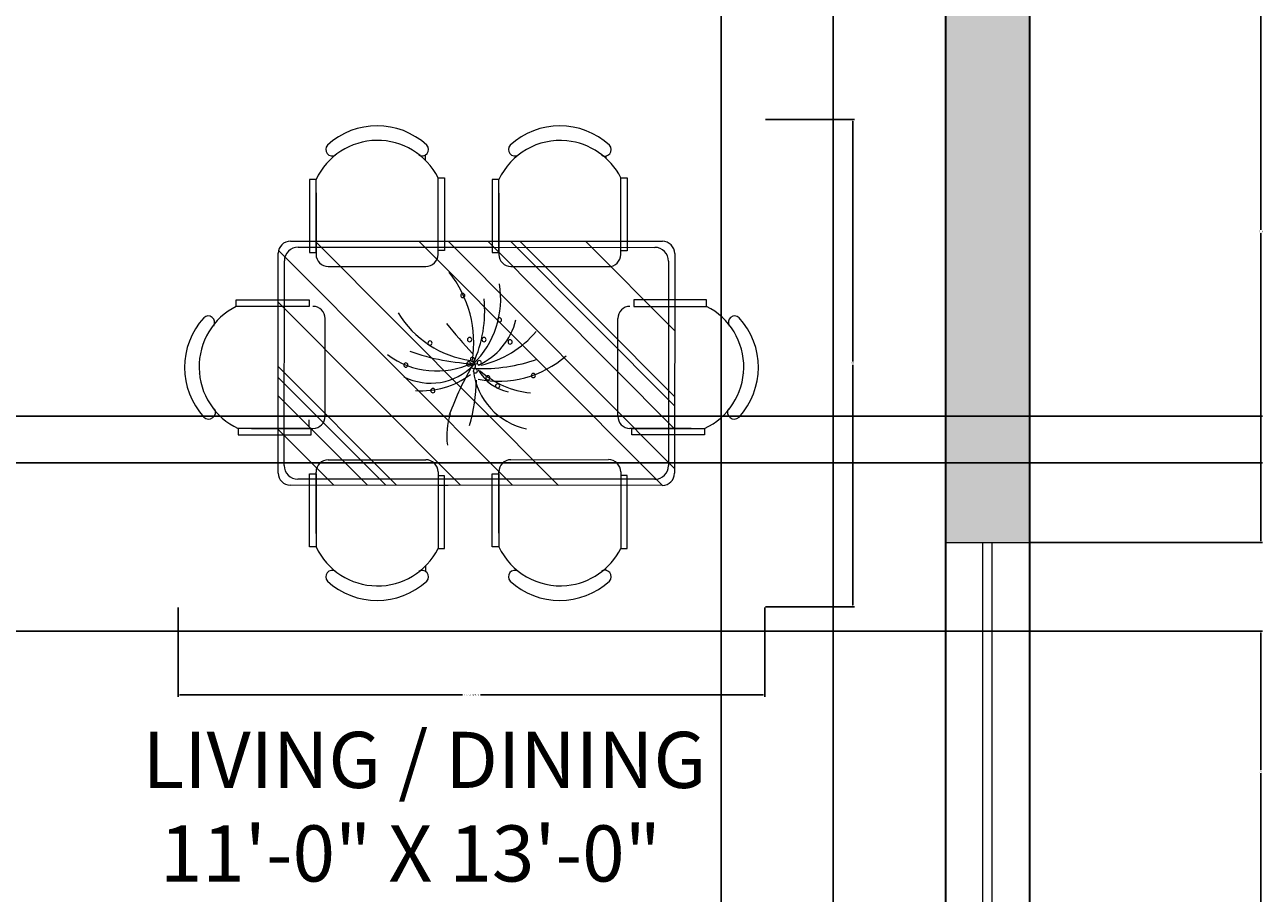
# Model space of a CAD drawing. Units: inches. Extents: x 126 to 477, y -70 to 465.
# Tile 4 of 5: x 344 to 477, y 195 to 288. Entities that reach past the tile are written whole.
import ezdxf

# ---------------------------------------------------------------- set-up
doc = ezdxf.new("R2010")
doc.units = ezdxf.units.IN
for name, color, linetype, lineweight in [('A-ANNO-DIMS', 2, 'Continuous', 18), ('A-AREA-IDEN', 7, 'Continuous', 20), ('A-FURN', 8, 'Continuous', 18), ('A-GLAZ', 4, 'Continuous', 18), ('A-WALL', 7, 'Continuous', 35), ('A-WALL-PATT', 252, 'Continuous', 13)]:
    doc.layers.add(name, color=color, linetype=linetype, lineweight=lineweight)
doc.styles.get("Standard").update_dxf_attribs({"font": 'arial.ttf'})
doc.dimstyles.get("Standard").update_dxf_attribs({"dimtxt": 0.18, "dimasz": 0.18, "dimexe": 0.18, "dimexo": 0.0625, "dimgap": 0.09, "dimtad": 0, "dimtih": 1, "dimtoh": 1, "dimdec": 4, "dimzin": 0, "dimdsep": 46, "dimtxsty": 'Standard', "dimcen": 0.09, "dimadec": 0, "dimazin": 0, "dimtfac": 1, "dimtdec": 4, "dimtofl": 0, "dimtmove": 0, "dimatfit": 3, "dimfxl": 1, "dimtolj": 1, "dimtzin": 0, "dimarcsym": 0})

# ---------------------------------------------------------------- blocks, each defined once
blk = doc.blocks.new('A$C6327331B')
for p, q in [((790.8, 678.3), (790.8, 696.4)), ((790.8, 678.3), (790.8, 696.4)), ((1381.3, 692.8), (1381.3, 686.2)), ((1381.3, 692.8), (1381.3, 686.2)), ((410.1, 615.8), (410, 377)), ((410.1, 615.8), (410, 377)), ((431.6, 615.8), (410.1, 615.8)), ((431.6, 615.8), (410.1, 615.8)), ((431.4, 376.9), (431.6, 615.8)), ((431.4, 376.9), (431.6, 615.8)), ((831.4, 382.9), (831.6, 621.7)), ((831.4, 382.9), (831.6, 621.7)), ((831.6, 621.7), (853, 621.7)), ((831.6, 621.7), (853, 621.7)), ((853, 621.7), (852.9, 382.9)), ((853, 621.7), (852.9, 382.9)), ((1009.3, 615.5), (1009.2, 376.7)), ((1009.3, 615.5), (1009.2, 376.7)), ((1030.7, 615.5), (1009.3, 615.5)), ((1030.7, 615.5), (1009.3, 615.5)), ((1030.6, 376.6), (1030.7, 615.5)), ((1030.6, 376.6), (1030.7, 615.5)), ((1430.6, 382.6), (1430.7, 621.4)), ((1430.6, 382.6), (1430.7, 621.4)), ((1430.7, 621.4), (1452.2, 621.4)), ((1430.7, 621.4), (1452.2, 621.4)), ((1452.2, 621.4), (1452, 382.6)), ((1452.2, 621.4), (1452, 382.6)), ((431.5, 571.8), (431.4, 370.8)), ((431.5, 571.8), (431.4, 370.8)), ((831.4, 370.6), (831.5, 571.6)), ((831.4, 370.6), (831.5, 571.6)), ((1030.7, 571.5), (1030.6, 370.5)), ((1030.7, 571.5), (1030.6, 370.5)), ((1430.6, 370.3), (1430.7, 571.3)), ((1430.6, 370.3), (1430.7, 571.3)), ((347.5, 414), (831.5, 413.8)), ((347.5, 414), (831.5, 413.8)), ((1226.3, -386.4), (428, 414)), ((1226.3, -386.4), (428, 414)), ((1567.1, -386.6), (768.8, 413.8)), ((1567.1, -386.6), (768.8, 413.8)), ((831.5, 413.8), (1567.5, 413.4)), ((1607.1, -331.3), (864.1, 413.8)), ((1607.1, -331.3), (864.1, 413.8)), ((1607.2, -200.8), (994.4, 413.7)), ((1607.2, -200.8), (994.4, 413.7)), ((1009.2, 413.7), (1567.5, 413.4)), ((1607.2, -125.5), (1069.5, 413.7)), ((1607.2, -125.5), (1069.5, 413.7)), ((1607.2, -95.4), (1099.6, 413.6)), ((1607.2, -95.4), (1099.6, 413.6)), ((1607.3, 120.5), (1315.1, 413.5)), ((1607.3, 120.5), (1315.1, 413.5)), ((1415.7, 413.4), (1415.7, 413.5)), ((1415.7, 413.4), (1415.7, 413.5)), ((307.1, -346), (307.5, 374)), ((307.1, -346), (307.5, 374)), ((1075.9, -386.3), (308.5, 383.1)), ((1075.9, -386.3), (308.5, 383.1)), ((372.5, 394), (831.4, 393.8)), ((372.5, 394), (1009.2, 393.7)), ((410, 377), (431.4, 376.9)), ((410, 377), (431.4, 376.9)), ((852.9, 382.9), (831.4, 382.9)), ((852.9, 382.9), (831.4, 382.9)), ((1009.2, 393.7), (1542.5, 393.4)), ((1009.2, 376.7), (1030.6, 376.6)), ((1009.2, 376.7), (1030.6, 376.6)), ((1452, 382.6), (1430.6, 382.6)), ((1452, 382.6), (1430.6, 382.6)), ((1607.5, 373.4), (1607.1, -346.6)), ((1607.5, 373.4), (1607.1, -346.6)), ((327.1, -321), (327.5, 349)), ((471.4, 330.8), (791.4, 330.6)), ((471.4, 330.8), (791.4, 330.6)), ((1070.6, 330.5), (1390.6, 330.3)), ((1070.6, 330.5), (1390.6, 330.3)), ((1587.5, 348.4), (1587.1, -321.6)), ((169.9, 221.5), (408.7, 221.6)), ((169.9, 221.5), (408.7, 221.6)), ((169.9, 200.1), (169.9, 221.5)), ((169.9, 200.1), (169.9, 221.5)), ((905.5, -386.3), (307.4, 213.5)), ((905.5, -386.3), (307.4, 213.5)), ((408.7, 221.6), (408.7, 200.2)), ((408.7, 221.6), (408.7, 200.2)), ((1473.3, 221.6), (1473.3, 200.2)), ((1473.3, 221.6), (1473.3, 200.2)), ((1712.1, 221.5), (1473.3, 221.6)), ((1712.1, 221.5), (1473.3, 221.6)), ((1712.1, 200.1), (1712.1, 221.5)), ((1712.1, 200.1), (1712.1, 221.5)), ((408.7, 200.2), (169.9, 200.1)), ((408.7, 200.2), (169.9, 200.1)), ((1473.3, 200.2), (1712.1, 200.1)), ((1473.3, 200.2), (1712.1, 200.1)), ((461.2, -159.8), (461, 160.2)), ((461.2, -159.8), (461, 160.2)), ((1420.8, -159.8), (1420.9, 160.2)), ((1420.8, -159.8), (1420.9, 160.2)), ((695.1, -386.2), (307.3, 2.7)), ((695.1, -386.2), (307.3, 2.7)), ((44.6, -20.2), (44.5, -20.1)), ((44.6, -20.2), (44.5, -20.1)), ((660, -386.1), (307.3, -32.5)), ((660, -386.1), (307.3, -32.5)), ((1837.4, -20.2), (1837.5, -20.1)), ((1837.4, -20.2), (1837.5, -20.1)), ((599.8, -386.1), (307.2, -92.7)), ((599.8, -386.1), (307.2, -92.7)), ((415.1, -199.8), (176.2, -199.9)), ((415.1, -199.8), (176.2, -199.9)), ((176.2, -199.9), (176.2, -221.3)), ((176.2, -199.9), (176.2, -221.3)), ((220.2, -199.9), (421.2, -199.8)), ((220.2, -199.9), (421.2, -199.8)), ((408.7, -193.6), (408.7, -172.1)), ((408.7, -193.6), (408.7, -172.1)), ((415.1, -221.2), (415.1, -199.8)), ((415.1, -221.2), (415.1, -199.8)), ((1661.8, -199.9), (1460.8, -199.8)), ((1661.8, -199.9), (1460.8, -199.8)), ((1466.9, -221.2), (1466.9, -199.8)), ((1466.9, -221.2), (1466.9, -199.8)), ((1466.9, -199.8), (1705.7, -199.9)), ((1466.9, -199.8), (1705.7, -199.9)), ((1705.7, -199.9), (1705.7, -221.3)), ((1705.7, -199.9), (1705.7, -221.3)), ((176.2, -221.3), (415.1, -221.2)), ((176.2, -221.3), (415.1, -221.2)), ((489.6, -386), (307.2, -203.2)), ((489.6, -386), (307.2, -203.2)), ((1705.7, -221.3), (1466.9, -221.2)), ((1705.7, -221.3), (1466.9, -221.2)), ((471.4, -302.7), (791.4, -302.5)), ((471.4, -302.7), (791.4, -302.5)), ((1070.6, -302.4), (1390.6, -302.2)), ((1070.6, -302.4), (1390.6, -302.2)), ((410.1, -587.7), (410, -348.9)), ((410.1, -587.7), (410, -348.9)), ((410, -348.9), (431.4, -348.9)), ((410, -348.9), (431.4, -348.9)), ((431.5, -543.7), (431.4, -342.7)), ((431.5, -543.7), (431.4, -342.7)), ((431.4, -348.9), (431.6, -587.7)), ((431.4, -348.9), (431.6, -587.7)), ((831.4, -342.5), (831.5, -543.5)), ((831.4, -342.5), (831.5, -543.5)), ((831.4, -354.8), (831.6, -593.6)), ((831.4, -354.8), (831.6, -593.6)), ((852.9, -354.8), (831.4, -354.8)), ((852.9, -354.8), (831.4, -354.8)), ((853, -593.6), (852.9, -354.8)), ((853, -593.6), (852.9, -354.8)), ((1009.2, -348.6), (1030.6, -348.5)), ((1009.2, -348.6), (1030.6, -348.5)), ((1009.3, -587.4), (1009.2, -348.6)), ((1009.3, -587.4), (1009.2, -348.6)), ((1030.7, -543.4), (1030.6, -342.4)), ((1030.7, -543.4), (1030.6, -342.4)), ((1030.6, -348.5), (1030.7, -587.4)), ((1030.6, -348.5), (1030.7, -587.4)), ((1430.6, -342.2), (1430.7, -543.2)), ((1430.6, -342.2), (1430.7, -543.2)), ((1430.6, -354.5), (1430.7, -593.3)), ((1430.6, -354.5), (1430.7, -593.3)), ((1452, -354.5), (1430.6, -354.5)), ((1452, -354.5), (1430.6, -354.5)), ((1452.2, -593.3), (1452, -354.5)), ((1452.2, -593.3), (1452, -354.5)), ((1567.1, -386.6), (347.1, -386)), ((1567.1, -386.6), (347.1, -386)), ((1542.1, -366.6), (372.1, -366)), ((831.5, -385.7), (864.1, -385.7)), ((831.5, -385.7), (864.1, -385.7)), ((1415.7, -385.3), (1415.7, -385.4)), ((1415.7, -385.3), (1415.7, -385.4)), ((431.6, -587.7), (410.1, -587.7)), ((431.6, -587.7), (410.1, -587.7)), ((831.6, -593.6), (853, -593.6)), ((831.6, -593.6), (853, -593.6)), ((1030.7, -587.4), (1009.3, -587.4)), ((1030.7, -587.4), (1009.3, -587.4)), ((1430.7, -593.3), (1452.2, -593.3)), ((1430.7, -593.3), (1452.2, -593.3)), ((790.8, -650.2), (790.8, -668.4)), ((790.8, -650.2), (790.8, -668.4)), ((1381.3, -664.7), (1381.3, -658.1)), ((1381.3, -664.7), (1381.3, -658.1))]:
    blk.add_line(p, q)
for centre, radius, start, end in [((631.5, 550.5), 241.3, 47.4691, 132.4721), ((631.5, 550.5), 241.3, 47.4691, 132.4721), ((1230.7, 550.2), 241.3, 47.4691, 132.4721), ((1230.7, 550.2), 241.3, 47.4691, 132.4721), ((633, 521.6), 222.4, 26.7656, 154.9369), ((633, 521.6), 222.4, 26.7656, 154.9369), ((1232.2, 521.3), 222.4, 84.4265, 154.9369), ((1232.2, 521.3), 222.4, 84.4265, 154.9369), ((1232.2, 521.3), 222.4, 26.7656, 84.4265), ((1232.2, 521.3), 222.4, 26.7656, 84.4265), ((484.3, 714.2), 21.2, 137.6497, 300.3412), ((484.3, 714.2), 21.2, 137.6497, 300.3412), ((779, 714), 21.2, 239.6, 42.2915), ((779, 714), 21.2, 239.6, 42.2915), ((1083.4, 713.9), 21.2, 137.6497, 300.3412), ((1083.4, 713.9), 21.2, 137.6497, 300.3412), ((1378.1, 713.7), 21.2, 239.6, 42.2915), ((1378.1, 713.7), 21.2, 239.6, 42.2915), ((347.5, 374), 40, 89.9706, 179.9706), ((347.5, 374), 40, 89.9706, 179.9706), ((1567.5, 373.4), 40, 359.9706, 89.9706), ((1567.5, 373.4), 40, 359.9706, 89.9706), ((372.5, 349), 45, 89.9706, 179.9706), ((471.4, 370.8), 40, 179.9706, 269.9706), ((471.4, 370.8), 40, 179.9706, 269.9706), ((791.4, 370.6), 40, 269.9706, 359.9706), ((791.4, 370.6), 40, 269.9706, 359.9706), ((1070.6, 370.5), 40, 179.9706, 269.9706), ((1070.6, 370.5), 40, 179.9706, 269.9706), ((1390.6, 370.3), 40, 269.9706, 359.9706), ((1390.6, 370.3), 40, 269.9706, 359.9706), ((1542.5, 348.4), 45, 359.9706, 89.9706), ((574.1, 79.9), 374.6, 351.2496, 38.2333), ((737.8, 225), 299.2, 314.4861, 9.3762), ((912.6, 235.7), 6.91, 0, 180), ((912.6, 235.7), 6.91, 180, 0), ((586.4, 182.9), 398.1, 335.0888, 5.9637), ((241.3, 0.1), 241.3, 137.5279, 222.5309), ((270.2, 1.6), 222.4, 116.8244, 244.9957), ((270.2, 1.6), 222.4, 116.8244, 244.9957), ((77.6, 147.4), 21.2, 329.6588, 132.3503), ((77.6, 147.4), 21.2, 329.6588, 132.3503), ((421, 160.2), 40, 0.0294, 90.0294), ((421, 160.2), 40, 0.0294, 90.0294), ((983.2, 350.8), 331, 211.315, 262.1378), ((1033, 155.9), 6.91, 0, 180), ((1460.9, 160.2), 40, 89.9706, 179.9706), ((1460.9, 160.2), 40, 89.9706, 179.9706), ((1611.7, 1.6), 222.4, 295.0043, 63.1756), ((1611.7, 1.6), 222.4, 295.0043, 63.1756), ((1804.4, 147.4), 21.2, 47.6497, 210.3412), ((1804.4, 147.4), 21.2, 47.6497, 210.3412), ((1640.7, 0.1), 241.3, 317.4691, 42.4721), ((1640.7, 0.1), 241.3, 317.4691, 42.4721), ((2460.3, 1443.6), 2062.1, 219.0488, 222.6799), ((873.8, 207.8), 219.3, 294.0956, 346.2953), ((1033, 155.9), 6.91, 180, 0), ((805, 79.9), 6.91, 0, 180), ((934.8, 91.3), 6.91, 0, 180), ((934.8, 91.3), 6.91, 180, 0), ((897.1, 334.6), 335.6, 283.0452, 319.7766), ((982.3, 91.3), 6.91, 0, 180), ((982.3, 91.3), 6.91, 180, 0), ((1067.8, 83.7), 6.91, 0, 180), ((1067.8, 83.7), 6.91, 180, 0), ((826.9, 258.5), 270.1, 233.3231, 295.7633), ((985.1, 750.7), 739.8, 250.5249, 267.8244), ((805, 79.9), 6.91, 180, 0), ((725.8, 7.7), 6.91, 0, 180), ((725.8, 7.7), 6.91, 180, 0), ((807.8, 143), 194.5, 242.9909, 315.9102), ((1747.6, -469.5), 933.6, 148.9873, 160.361), ((931.7, 11.5), 6.91, 0, 180), ((931.7, 11.5), 6.91, 180, 0), ((944.3, 26.7), 6.91, 0, 180), ((944.3, 26.7), 6.91, 180, 0), ((947.5, 3.9), 6.91, 0, 180), ((947.5, 3.9), 6.91, 180, 0), ((970.7, 574.8), 578.8, 268.3286, 288.729), ((966.5, 15.3), 6.91, 0, 180), ((966.5, 15.3), 6.91, 180, 0), ((1030.3, 292.7), 337.4, 258.5516, 310.9815), ((776.7, 191.6), 268.2, 265.8741, 306.9558), ((953.8, -11.3), 6.91, 0, 180), ((953.8, -11.3), 6.91, 180, 0), ((1167.7, 15.7), 221.9, 186.9904, 258.0284), ((1090.6, 62.7), 145.4, 208.8901, 258.4579), ((1166.2, 212.9), 298.2, 228.7581, 263.8624), ((995, -34.1), 6.91, 0, 180), ((995, -34.1), 6.91, 180, 0), ((1143.8, -26.5), 6.91, 0, 180), ((1143.8, -26.5), 6.91, 180, 0), ((814.5, -75.9), 6.91, 0, 180), ((814.5, -75.9), 6.91, 180, 0), ((392.7, -33), 564.4, 343.8561, 359.1105), ((1026.7, -60.7), 6.91, 0, 180), ((1026.7, -60.7), 6.91, 180, 0), ((79, -146.7), 22.5, 226.3776, 29.8882), ((79, -146.7), 22.5, 226.3776, 29.8882), ((421.2, -159.8), 40, 270.0294, 0.0294), ((421.2, -159.8), 40, 270.0294, 0.0294), ((1112.9, -226), 252.6, 162.9456, 186.4814), ((1460.8, -159.8), 40, 179.9706, 269.9706), ((1460.8, -159.8), 40, 179.9706, 269.9706), ((1803, -146.7), 22.5, 150.1118, 313.6224), ((1803, -146.7), 22.5, 150.1118, 313.6224), ((372.1, -321), 45, 179.9706, 269.9706), ((471.4, -342.7), 40, 90.0294, 180.0294), ((471.4, -342.7), 40, 90.0294, 180.0294), ((791.4, -342.5), 40, 0.0294, 90.0294), ((791.4, -342.5), 40, 0.0294, 90.0294), ((1070.6, -342.4), 40, 90.0294, 180.0294), ((1070.6, -342.4), 40, 90.0294, 180.0294), ((1390.6, -342.2), 40, 0.0294, 90.0294), ((1390.6, -342.2), 40, 0.0294, 90.0294), ((1542.1, -321.6), 45, 269.9706, 359.9706), ((347.1, -346), 40, 179.9706, 269.9706), ((347.1, -346), 40, 179.9706, 269.9706), ((1567.1, -346.6), 40, 269.9706, 359.9706), ((1567.1, -346.6), 40, 269.9706, 359.9706), ((633, -493.5), 222.4, 205.0631, 333.2344), ((633, -493.5), 222.4, 205.0631, 333.2344), ((1232.2, -493.2), 222.4, 205.0631, 275.5735), ((1232.2, -493.2), 222.4, 205.0631, 275.5735), ((1232.2, -493.2), 222.4, 275.5735, 333.2344), ((1232.2, -493.2), 222.4, 275.5735, 333.2344), ((484.3, -686.1), 21.2, 59.6588, 222.3503), ((484.3, -686.1), 21.2, 59.6588, 222.3503), ((779, -686), 21.2, 317.7085, 120.4), ((779, -686), 21.2, 317.7085, 120.4), ((1083.4, -685.8), 21.2, 59.6588, 222.3503), ((1083.4, -685.8), 21.2, 59.6588, 222.3503), ((1378.1, -685.6), 21.2, 317.7085, 120.4), ((1378.1, -685.6), 21.2, 317.7085, 120.4), ((631.5, -522.4), 241.3, 227.5279, 312.5309), ((631.5, -522.4), 241.3, 227.5279, 312.5309), ((1230.7, -522.1), 241.3, 227.5279, 312.5309), ((1230.7, -522.1), 241.3, 227.5279, 312.5309)]:
    blk.add_arc(centre, radius, start, end)
at = {"width": 0.8, "flags": 9}
for tag in ['XSIZE', 'YSIZE']:
    blk.add_attdef(tag, (945.2, 11.4), '', height=0.23, rotation=180, dxfattribs=at)
blk = doc.blocks.new('WIN-72IN')
for p, q in [((0, 0), (0, 9)), ((72, 0), (72, 9)), ((72, 5), (0, 5)), ((72, 4), (0, 4))]:
    blk.add_line(p, q)
blk = doc.blocks.new('*D27')
at = {"layer": 'A-ANNO-DIMS', "color": 0, "lineweight": -2, "transparency": 16777216}
for p, q in [((360.43, 225.42), (360.43, 215.89)), ((423.2, 225.42), (423.2, 215.89)), ((360.61, 216.07), (390.85, 216.07)), ((423.02, 216.07), (392.79, 216.07))]:
    blk.add_line(p, q, dxfattribs=at)
at = {"layer": 'A-ANNO-DIMS', "color": 0, "transparency": 16777216}
for points in [[(360.61, 216.1), (360.61, 216.04), (360.43, 216.07)], [(423.02, 216.1), (423.02, 216.04), (423.2, 216.07)]]:
    blk.add_solid(points, dxfattribs=at)
at = {"layer": 'Defpoints', "color": 0, "transparency": 16777216}
for p in [(360.43, 225.48), (423.2, 225.48), (423.2, 216.07)]:
    blk.add_point(p, dxfattribs=at)
at = {"layer": 'A-ANNO-DIMS', "color": 0, "transparency": 16777216, "insert": (391.82, 216.07), "char_height": 0.18, "attachment_point": 5}
blk.add_mtext('\\A1;DINING SET 63', dxfattribs=at)
blk = doc.blocks.new('*D28')
at = {"layer": 'A-ANNO-DIMS', "color": 0, "lineweight": -2, "transparency": 16777216}
for p, q in [((423.27, 277.6), (432.8, 277.6)), ((432.62, 277.42), (432.62, 251.72)), ((432.62, 225.66), (432.62, 251.36)), ((423.27, 225.48), (432.8, 225.48))]:
    blk.add_line(p, q, dxfattribs=at)
at = {"layer": 'A-ANNO-DIMS', "color": 0, "transparency": 16777216}
for points in [[(432.59, 277.42), (432.65, 277.42), (432.62, 277.6)], [(432.59, 225.66), (432.65, 225.66), (432.62, 225.48)]]:
    blk.add_solid(points, dxfattribs=at)
at = {"layer": 'Defpoints', "color": 0, "transparency": 16777216}
for p in [(423.2, 277.6), (432.62, 277.6), (423.2, 225.48)]:
    blk.add_point(p, dxfattribs=at)
at = {"layer": 'A-ANNO-DIMS', "color": 0, "transparency": 16777216, "insert": (432.62, 251.54), "char_height": 0.18, "attachment_point": 5}
blk.add_mtext('\\A1;52', dxfattribs=at)
blk = doc.blocks.new('*D32')
at = {"layer": 'A-ANNO-DIMS', "color": 0, "lineweight": -2, "transparency": 16777216}
for p, q in [((430.53, 430.82), (430.53, -70.05)), ((442.53, 430.82), (442.53, -70.05)), ((430.71, -69.87), (436.32, -69.87)), ((442.35, -69.87), (436.74, -69.87))]:
    blk.add_line(p, q, dxfattribs=at)
at = {"layer": 'A-ANNO-DIMS', "color": 0, "transparency": 16777216}
for points in [[(430.71, -69.84), (430.71, -69.9), (430.53, -69.87)], [(442.35, -69.84), (442.35, -69.9), (442.53, -69.87)]]:
    blk.add_solid(points, dxfattribs=at)
at = {"layer": 'Defpoints', "color": 0, "transparency": 16777216}
for p in [(430.53, 430.88), (442.53, 430.88), (442.53, -69.87)]:
    blk.add_point(p, dxfattribs=at)
at = {"layer": 'A-ANNO-DIMS', "color": 0, "transparency": 16777216, "insert": (436.53, -69.87), "char_height": 0.18, "attachment_point": 5}
blk.add_mtext('\\A1;12', dxfattribs=at)
blk = doc.blocks.new('*D37')
at = {"layer": 'A-ANNO-DIMS', "color": 0, "lineweight": -2, "transparency": 16777216}
for p, q in [((442.6, 298.88), (476.46, 298.88)), ((476.28, 298.7), (476.28, 265.81)), ((476.28, 232.56), (476.28, 265.45)), ((451.6, 232.38), (476.46, 232.38))]:
    blk.add_line(p, q, dxfattribs=at)
at = {"layer": 'A-ANNO-DIMS', "color": 0, "transparency": 16777216}
for points in [[(476.25, 298.7), (476.31, 298.7), (476.28, 298.88)], [(476.25, 232.56), (476.31, 232.56), (476.28, 232.38)]]:
    blk.add_solid(points, dxfattribs=at)
at = {"layer": 'Defpoints', "color": 0, "transparency": 16777216}
for p in [(442.53, 298.88), (476.28, 298.88), (451.53, 232.38)]:
    blk.add_point(p, dxfattribs=at)
at = {"layer": 'A-ANNO-DIMS', "color": 0, "transparency": 16777216, "insert": (476.28, 265.63), "char_height": 0.18, "attachment_point": 5}
blk.add_mtext('\\A1;66.5', dxfattribs=at)
blk = doc.blocks.new('*D48')
at = {"layer": 'A-ANNO-DIMS', "color": 0, "lineweight": -2, "transparency": 16777216}
for p, q in [((418.53, 298.82), (418.53, -70.05)), ((442.53, 298.82), (442.53, -70.05)), ((418.71, -69.87), (430.31, -69.87)), ((442.35, -69.87), (430.75, -69.87))]:
    blk.add_line(p, q, dxfattribs=at)
at = {"layer": 'A-ANNO-DIMS', "color": 0, "transparency": 16777216}
for points in [[(418.71, -69.84), (418.71, -69.9), (418.53, -69.87)], [(442.35, -69.84), (442.35, -69.9), (442.53, -69.87)]]:
    blk.add_solid(points, dxfattribs=at)
at = {"layer": 'Defpoints', "color": 0, "transparency": 16777216}
for p in [(418.53, 298.88), (442.53, 298.88), (442.53, -69.87)]:
    blk.add_point(p, dxfattribs=at)
at = {"layer": 'A-ANNO-DIMS', "color": 0, "transparency": 16777216, "insert": (430.53, -69.87), "char_height": 0.18, "attachment_point": 5}
blk.add_mtext('\\A1;24', dxfattribs=at)
blk = doc.blocks.new('*D51')
at = {"layer": 'A-ANNO-DIMS', "color": 0, "lineweight": -2, "transparency": 16777216}
for p, q in [((293.6, 222.88), (476.46, 222.88)), ((476.28, 222.7), (476.28, 208.06)), ((476.28, 193.06), (476.28, 207.7)), ((293.6, 192.88), (476.46, 192.88))]:
    blk.add_line(p, q, dxfattribs=at)
at = {"layer": 'A-ANNO-DIMS', "color": 0, "transparency": 16777216}
for points in [[(476.25, 222.7), (476.31, 222.7), (476.28, 222.88)], [(476.25, 193.06), (476.31, 193.06), (476.28, 192.88)]]:
    blk.add_solid(points, dxfattribs=at)
at = {"layer": 'Defpoints', "color": 0, "transparency": 16777216}
for p in [(293.53, 222.88), (476.28, 222.88), (293.53, 192.88)]:
    blk.add_point(p, dxfattribs=at)
at = {"layer": 'A-ANNO-DIMS', "color": 0, "transparency": 16777216, "insert": (476.28, 207.88), "char_height": 0.18, "attachment_point": 5}
blk.add_mtext('\\A1;30', dxfattribs=at)
blk = doc.blocks.new('*D54')
at = {"layer": 'A-ANNO-DIMS', "color": 0, "lineweight": -2, "transparency": 16777216}
for p, q in [((288.6, 245.88), (476.46, 245.88)), ((476.28, 245.7), (476.28, 243.56)), ((476.28, 241.06), (476.28, 243.2)), ((288.6, 240.88), (476.46, 240.88))]:
    blk.add_line(p, q, dxfattribs=at)
at = {"layer": 'A-ANNO-DIMS', "color": 0, "transparency": 16777216}
for points in [[(476.25, 245.7), (476.31, 245.7), (476.28, 245.88)], [(476.25, 241.06), (476.31, 241.06), (476.28, 240.88)]]:
    blk.add_solid(points, dxfattribs=at)
at = {"layer": 'Defpoints', "color": 0, "transparency": 16777216}
for p in [(288.53, 245.88), (476.28, 245.88), (288.53, 240.88)]:
    blk.add_point(p, dxfattribs=at)
at = {"layer": 'A-ANNO-DIMS', "color": 0, "transparency": 16777216, "insert": (476.28, 243.38), "char_height": 0.18, "attachment_point": 5}
blk.add_mtext('\\A1;5', dxfattribs=at)

msp = doc.modelspace()

# ---------------------------------------------------------------- hatches: boundary and pattern name
at = {"layer": 'A-WALL-PATT'}
h = msp.add_hatch(color=256, dxfattribs=at)
h.dxf.hatch_style = 1
h.paths.add_polyline_path([(451.5333, 439.8806), (430.5333, 439.8806), (430.5333, 430.8806), (442.5333, 430.8806), (442.5333, 298.8806), (382.5333, 298.8806), (382.5333, 293.8806), (442.5333, 293.8806), (442.5333, 232.3806), (451.5333, 232.3806)])

# ---------------------------------------------------------------- linework, layer by layer
at = {"layer": 'A-WALL'}
for p, q in [((451.5333, 439.8806), (451.5333, -45.1194)), ((442.5333, 293.8806), (442.5333, 98.8806))]:
    msp.add_line(p, q, dxfattribs=at)

# ---------------------------------------------------------------- block references
at = {"layer": 'A-FURN', "xscale": 0.032620503702758, "yscale": 0.032620503702758, "zscale": 0.032620503702758}
msp.add_blockref('A$C6327331B', (361.1227, 251.0846), dxfattribs=at)
at = {"layer": 'A-GLAZ', "rotation": 269.9999999999998}
msp.add_blockref('WIN-72IN', (442.5333, 232.3806), dxfattribs=at)

# ---------------------------------------------------------------- texts
at = {"layer": 'A-AREA-IDEN', "insert": (356.6451, 212.1317), "char_height": 6, "attachment_point": 1}
msp.add_mtext_dynamic_manual_height_columns('LIVING / DINING\\P 11\'-0" X 13\'-0"', width=74.074101, gutter_width=12.5, heights=[0], dxfattribs=at)

# ---------------------------------------------------------------- dimensions: what is measured, and where the dimension line sits
at = {"layer": 'A-ANNO-DIMS'}
for p1, p2, picture, middle in [((430.5333, 430.8806), (442.5333, 430.8806), '*D32', (436.5333, -69.8694)), ((418.5333, 298.8806), (442.5333, 298.8806), '*D48', (430.5333, -69.8694))]:
    dim = msp.add_linear_dim(base=(442.5333, -69.8694), p1=p1, p2=p2, dimstyle='Standard', override={"dimdec": 0, "dimlfac": 1, "dimrnd": 0, "dimzin": 0, "dimdsep": 46, "dimlunit": 2}, dxfattribs=at)
    dim.commit()
    dim.dimension.update_dxf_attribs({"geometry": picture, "text_midpoint": middle})
for base, p1, p2, override, picture, middle in [((476.2833, 298.8806), (451.5333, 232.3806), (442.5333, 298.8806), {"dimdec": 1, "dimlfac": 1, "dimrnd": 0, "dimzin": 0, "dimdsep": 46, "dimlunit": 2}, '*D37', (476.2833, 265.6306)), ((432.6197, 277.6043), (423.2039, 225.4813), (423.2039, 277.6043), {"dimdec": 0, "dimlfac": 1, "dimrnd": 0, "dimzin": 0, "dimdsep": 46, "dimlunit": 2}, '*D28', (432.6197, 251.5428)), ((476.2833, 245.8806), (288.5333, 240.8806), (288.5333, 245.8806), {"dimdec": 0, "dimlfac": 1, "dimrnd": 0, "dimzin": 0, "dimdsep": 46, "dimlunit": 2}, '*D54', (476.2833, 243.3806)), ((476.2833, 222.8806), (293.5333, 192.8806), (293.5333, 222.8806), {"dimdec": 0, "dimlfac": 1, "dimrnd": 0, "dimzin": 0, "dimdsep": 46, "dimlunit": 2}, '*D51', (476.2833, 207.8806))]:
    dim = msp.add_linear_dim(base=base, p1=p1, p2=p2, angle=90, dimstyle='Standard', override=override, dxfattribs=at)
    dim.commit()
    dim.dimension.update_dxf_attribs({"geometry": picture, "text_midpoint": middle})
dim = msp.add_linear_dim(base=(423.2039, 216.0655), p1=(360.4321, 225.4813), p2=(423.2039, 225.4813), text='DINING SET <>', dimstyle='Standard', override={"dimdec": 0, "dimlfac": 1, "dimrnd": 0, "dimzin": 0, "dimdsep": 46, "dimlunit": 2}, dxfattribs=at)
dim.commit()
dim.dimension.update_dxf_attribs({"geometry": '*D27', "text_midpoint": (391.818, 216.0655)})

doc.saveas('drawing.dxf')
